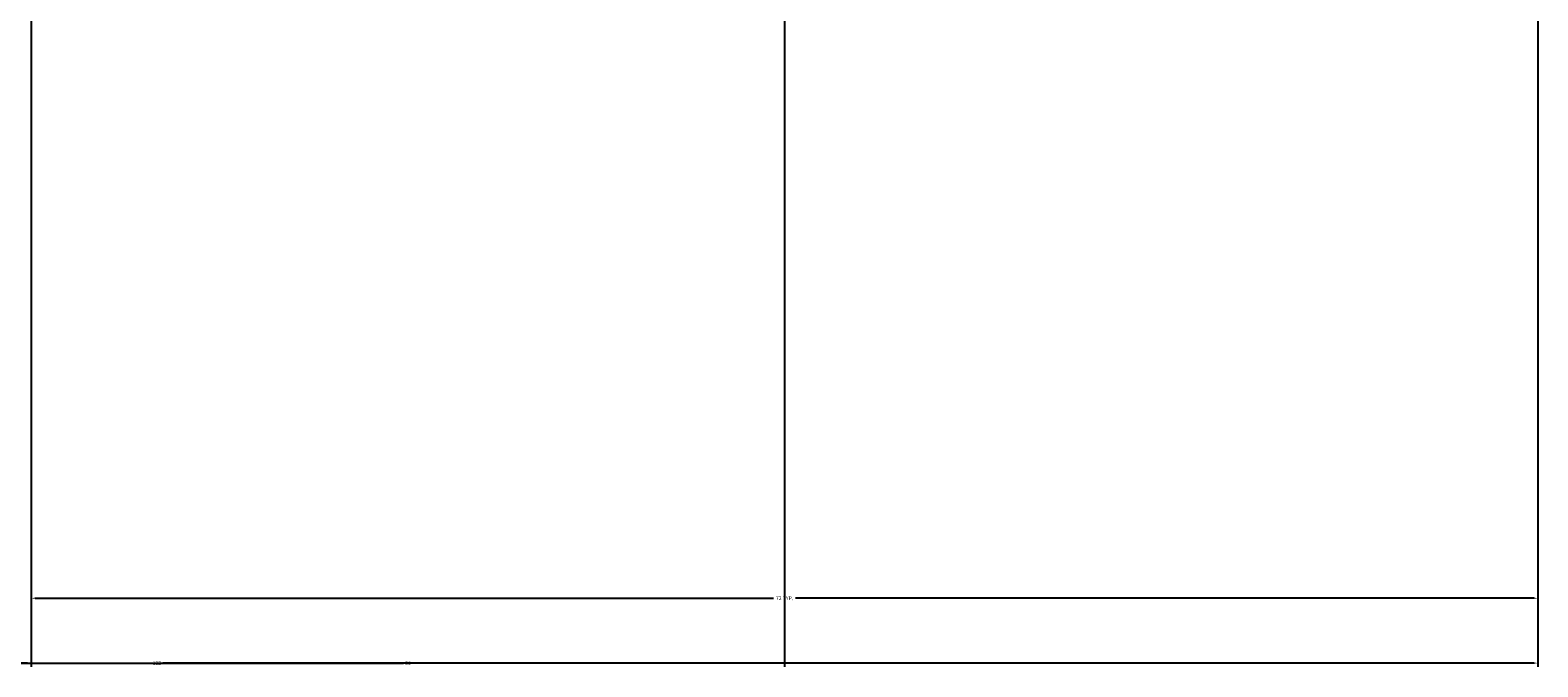
# Model space of a CAD drawing. Units: feet. Extents: x 1654 to 2985, y 1348 to 2230.
# Tile 18 of 53: x 2130 to 2202, y 1534 to 1565. Entities that reach past the tile are written whole.
import ezdxf

# ---------------------------------------------------------------- set-up
doc = ezdxf.new("R2010")
doc.units = ezdxf.units.FT
doc.layers.add('A-ANNO-DIMS', color=2, linetype='Continuous', lineweight=18)
doc.styles.get("Standard").update_dxf_attribs({"font": 'arial.ttf'})
doc.dimstyles.get("Standard").update_dxf_attribs({"dimtxt": 0.18, "dimasz": 0.18, "dimexe": 0.18, "dimexo": 0.0625, "dimgap": 0.09, "dimtad": 0, "dimtih": 1, "dimtoh": 1, "dimdec": 4, "dimzin": 0, "dimdsep": 46, "dimtxsty": 'Standard', "dimcen": 0.09, "dimadec": 0, "dimazin": 0, "dimtfac": 1, "dimtdec": 4, "dimtofl": 0, "dimtmove": 0, "dimatfit": 3, "dimfxl": 1, "dimtolj": 1, "dimtzin": 0, "dimarcsym": 0})

# ---------------------------------------------------------------- blocks, each defined once
blk = doc.blocks.new('*D73')
at = {"layer": 'A-ANNO-DIMS', "color": 0, "lineweight": -2, "transparency": 16777216}
for p, q in [((2130.092, 1565.192), (2130.092, 1537.175)), ((2202.092, 1565.192), (2202.092, 1537.175)), ((2130.272, 1537.355), (2165.565, 1537.355)), ((2201.912, 1537.355), (2166.62, 1537.355))]:
    blk.add_line(p, q, dxfattribs=at)
at = {"layer": 'A-ANNO-DIMS', "color": 0, "transparency": 16777216}
for points in [[(2130.272, 1537.385), (2130.272, 1537.325), (2130.092, 1537.355)], [(2201.912, 1537.385), (2201.912, 1537.325), (2202.092, 1537.355)]]:
    blk.add_solid(points, dxfattribs=at)
at = {"layer": 'Defpoints', "color": 0, "transparency": 16777216}
for p in [(2130.092, 1565.255), (2202.092, 1565.255), (2202.092, 1537.355)]:
    blk.add_point(p, dxfattribs=at)
at = {"layer": 'A-ANNO-DIMS', "color": 0, "transparency": 16777216, "insert": (2166.092, 1537.355), "char_height": 0.18, "attachment_point": 5}
blk.add_mtext('\\A1;72 TYP.', dxfattribs=at)
blk = doc.blocks.new('*D80')
at = {"layer": 'A-ANNO-DIMS', "color": 0, "lineweight": -2, "transparency": 16777216}
for p, q in [((2070.092, 2039.192), (2070.092, 1534.075)), ((2202.092, 2039.192), (2202.092, 1534.075)), ((2070.272, 1534.255), (2135.813, 1534.255)), ((2201.912, 1534.255), (2136.372, 1534.255))]:
    blk.add_line(p, q, dxfattribs=at)
at = {"layer": 'A-ANNO-DIMS', "color": 0, "transparency": 16777216}
for points in [[(2070.272, 1534.285), (2070.272, 1534.225), (2070.092, 1534.255)], [(2201.912, 1534.285), (2201.912, 1534.225), (2202.092, 1534.255)]]:
    blk.add_solid(points, dxfattribs=at)
at = {"layer": 'Defpoints', "color": 0, "transparency": 16777216}
for p in [(2070.092, 2039.255), (2202.092, 2039.255), (2202.092, 1534.255)]:
    blk.add_point(p, dxfattribs=at)
at = {"layer": 'A-ANNO-DIMS', "color": 0, "transparency": 16777216, "insert": (2136.092, 1534.255), "char_height": 0.18, "attachment_point": 5}
blk.add_mtext('\\A1;132', dxfattribs=at)
blk = doc.blocks.new('*D99')
at = {"layer": 'A-ANNO-DIMS', "color": 0, "lineweight": -2, "transparency": 16777216}
for p, q in [((2166.092, 1746.692), (2166.092, 1534.075)), ((2130.092, 1742.192), (2130.092, 1534.075)), ((2130.272, 1534.255), (2147.874, 1534.255)), ((2165.912, 1534.255), (2148.311, 1534.255))]:
    blk.add_line(p, q, dxfattribs=at)
at = {"layer": 'A-ANNO-DIMS', "color": 0, "transparency": 16777216}
for points in [[(2130.272, 1534.285), (2130.272, 1534.225), (2130.092, 1534.255)], [(2165.912, 1534.285), (2165.912, 1534.225), (2166.092, 1534.255)]]:
    blk.add_solid(points, dxfattribs=at)
at = {"layer": 'Defpoints', "color": 0, "transparency": 16777216}
for p in [(2166.092, 1746.755), (2130.092, 1742.255), (2166.092, 1534.255)]:
    blk.add_point(p, dxfattribs=at)
at = {"layer": 'A-ANNO-DIMS', "color": 0, "transparency": 16777216, "insert": (2148.092, 1534.255), "char_height": 0.18, "attachment_point": 5}
blk.add_mtext('\\A1;36', dxfattribs=at)
blk = doc.blocks.new('*D103')
at = {"layer": 'A-ANNO-DIMS', "color": 0, "lineweight": -2, "transparency": 16777216}
for p, q in [((2070.092, 1661.192), (2070.092, 1534.075)), ((2130.092, 1565.192), (2130.092, 1534.075)), ((2070.272, 1534.255), (2099.873, 1534.255)), ((2129.912, 1534.255), (2100.312, 1534.255))]:
    blk.add_line(p, q, dxfattribs=at)
at = {"layer": 'A-ANNO-DIMS', "color": 0, "transparency": 16777216}
for points in [[(2070.272, 1534.285), (2070.272, 1534.225), (2070.092, 1534.255)], [(2129.912, 1534.285), (2129.912, 1534.225), (2130.092, 1534.255)]]:
    blk.add_solid(points, dxfattribs=at)
at = {"layer": 'Defpoints', "color": 0, "transparency": 16777216}
for p in [(2070.092, 1661.255), (2130.092, 1565.255), (2130.092, 1534.255)]:
    blk.add_point(p, dxfattribs=at)
at = {"layer": 'A-ANNO-DIMS', "color": 0, "transparency": 16777216, "insert": (2100.092, 1534.255), "char_height": 0.18, "attachment_point": 5}
blk.add_mtext('\\A1;60', dxfattribs=at)

msp = doc.modelspace()

# ---------------------------------------------------------------- dimensions: what is measured, and where the dimension line sits
at = {"layer": 'A-ANNO-DIMS'}
for base, p1, p2, picture, middle in [((2202.0924, 1534.2549), (2070.0924, 2039.2549), (2202.0924, 2039.2549), '*D80', (2136.0924, 1534.2549)), ((2166.0924, 1534.2549), (2130.0924, 1742.2549), (2166.0924, 1746.7549), '*D99', (2148.0924, 1534.2549)), ((2130.0924, 1534.2549), (2070.0924, 1661.2549), (2130.0924, 1565.2549), '*D103', (2100.0924, 1534.2549))]:
    dim = msp.add_linear_dim(base=base, p1=p1, p2=p2, dimstyle='Standard', override={"dimdec": 0, "dimlfac": 1, "dimrnd": 0, "dimzin": 0, "dimdsep": 46, "dimlunit": 2}, dxfattribs=at)
    dim.commit()
    dim.dimension.update_dxf_attribs({"geometry": picture, "text_midpoint": middle})
dim = msp.add_linear_dim(base=(2202.0924, 1537.3549), p1=(2130.0924, 1565.2549), p2=(2202.0924, 1565.2549), text='<> TYP.', dimstyle='Standard', override={"dimdec": 0, "dimlfac": 1, "dimrnd": 0, "dimzin": 0, "dimdsep": 46, "dimlunit": 2}, dxfattribs=at)
dim.commit()
dim.dimension.update_dxf_attribs({"geometry": '*D73', "text_midpoint": (2166.0924, 1537.3549)})

doc.saveas('drawing.dxf')
